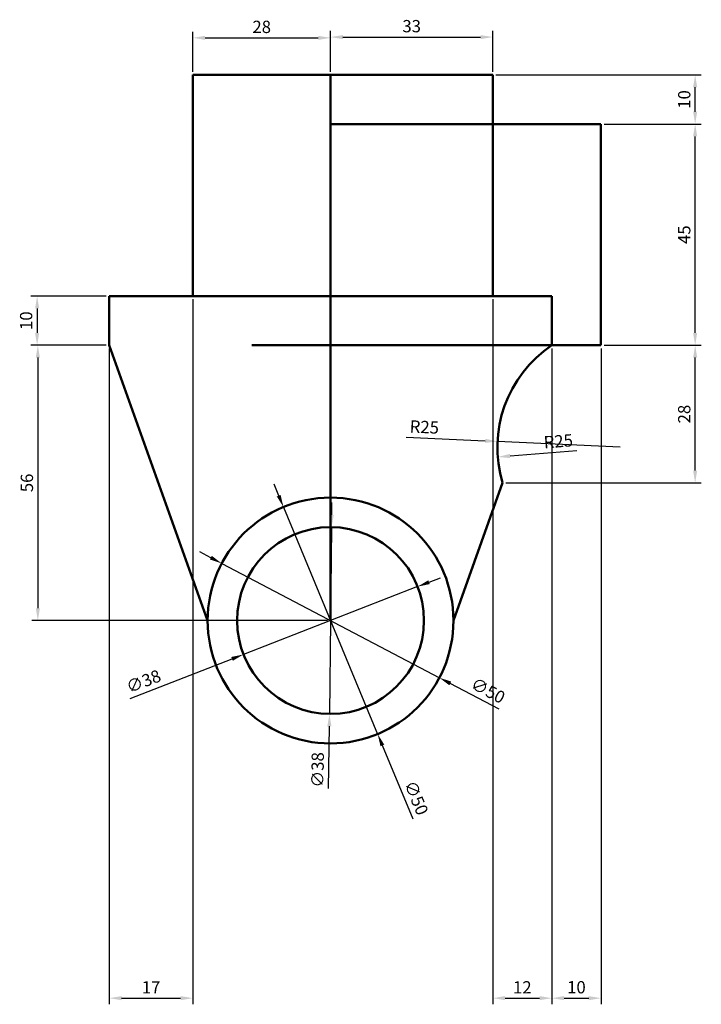
# Model space of a CAD drawing. Units: millimetres. Extents: x 2172 to 2566, y 897 to 1244.
# Tile 3 of 3: x 2427 to 2566, y 906 to 1106. Entities that reach past the tile are written whole.
import ezdxf

# ---------------------------------------------------------------- set-up
doc = ezdxf.new("R2010")
doc.units = ezdxf.units.MM
doc.layers.add('M-DIMS', color=2, linetype='Continuous', lineweight=25)
doc.layers.add('M-OUTL', color=7, linetype='Continuous', lineweight=50)
doc.styles.get("Standard").update_dxf_attribs({"font": 'arial.ttf'})
doc.dimstyles.new('ISO-25', dxfattribs={"dimtxt": 2.5, "dimasz": 2.5, "dimexe": 1.25, "dimexo": 0.625, "dimtad": 1, "dimtxsty": 'Standard', "dimcen": 2.5, "dimadec": 0, "dimazin": 0, "dimtfac": 1, "dimtmove": 0, "dimatfit": 3, "dimfxl": 1, "dimarcsym": 0})

# ---------------------------------------------------------------- blocks, each defined once
blk = doc.blocks.new('*D3')
at = {"layer": 'Defpoints', "color": 0, "transparency": 16777216}
for p in [(2507.9, 990.53), (2472.49, 976.73)]:
    blk.add_point(p, dxfattribs=at)
at = {"layer": 'M-DIMS', "color": 0, "lineweight": -2, "transparency": 16777216}
for p, q in [((2510.23, 991.43), (2512.56, 992.34)), ((2507.9, 990.53), (2472.49, 976.73)), ((2449.48, 967.76), (2470.16, 975.82))]:
    blk.add_line(p, q, dxfattribs=at)
at = {"layer": 'M-DIMS', "color": 0, "transparency": 16777216}
for points in [[(2510.08, 991.82), (2510.38, 991.05), (2507.9, 990.53)], [(2470.01, 976.21), (2470.32, 975.44), (2472.49, 976.73)]]:
    blk.add_solid(points, dxfattribs=at)
at = {"layer": 'M-DIMS', "color": 0, "transparency": 16777216, "insert": (2452.28, 970.97), "char_height": 2.5, "attachment_point": 5, "rotation": 21.2859}
blk.add_mtext('∅38', dxfattribs=at)
blk = doc.blocks.new('*D4')
at = {"layer": 'Defpoints', "color": 0, "transparency": 16777216}
for p in [(2468.07, 995.25), (2512.33, 972)]:
    blk.add_point(p, dxfattribs=at)
at = {"layer": 'M-DIMS', "color": 0, "lineweight": -2, "transparency": 16777216}
for p, q in [((2465.85, 996.42), (2463.64, 997.58)), ((2468.07, 995.25), (2512.33, 972)), ((2524.5, 965.61), (2514.54, 970.84))]:
    blk.add_line(p, q, dxfattribs=at)
at = {"layer": 'M-DIMS', "color": 0, "transparency": 16777216}
for points in [[(2466.05, 996.79), (2465.66, 996.05), (2468.07, 995.25)], [(2514.74, 971.21), (2514.35, 970.47), (2512.33, 972)]]:
    blk.add_solid(points, dxfattribs=at)
at = {"layer": 'M-DIMS', "color": 0, "transparency": 16777216, "insert": (2522.08, 969.11), "char_height": 2.5, "attachment_point": 5, "rotation": 332.2866}
blk.add_mtext('∅50', dxfattribs=at)
blk = doc.blocks.new('*D5')
at = {"layer": 'Defpoints', "color": 0, "transparency": 16777216}
for p in [(2549.13, 1018.87), (2524.2, 1016.9)]:
    blk.add_point(p, dxfattribs=at)
at = {"layer": 'M-DIMS', "color": 0, "lineweight": -2, "transparency": 16777216}
blk.add_line((2540.29, 1018.17), (2526.7, 1017.1), dxfattribs=at)
at = {"layer": 'M-DIMS', "color": 0, "transparency": 16777216}
blk.add_solid([(2526.66, 1017.51), (2526.73, 1016.68), (2524.2, 1016.9)], dxfattribs=at)
at = {"layer": 'M-DIMS', "color": 0, "transparency": 16777216, "insert": (2536.54, 1019.78), "char_height": 2.5, "attachment_point": 5, "rotation": 4.5166}
blk.add_mtext('R25', dxfattribs=at)
blk = doc.blocks.new('*D6')
at = {"layer": 'Defpoints', "color": 0, "transparency": 16777216}
for p in [(2445.2, 1039.63), (2430.67, 983.63), (2490.2, 983.63)]:
    blk.add_point(p, dxfattribs=at)
at = {"layer": 'M-DIMS', "color": 0, "lineweight": -2, "transparency": 16777216}
for p, q in [((2444.57, 1039.63), (2429.42, 1039.63)), ((2430.67, 1037.13), (2430.67, 986.13)), ((2489.57, 983.63), (2429.42, 983.63))]:
    blk.add_line(p, q, dxfattribs=at)
at = {"layer": 'M-DIMS', "color": 0, "transparency": 16777216}
for points in [[(2430.26, 1037.13), (2431.09, 1037.13), (2430.67, 1039.63)], [(2430.26, 986.13), (2431.09, 986.13), (2430.67, 983.63)]]:
    blk.add_solid(points, dxfattribs=at)
at = {"layer": 'M-DIMS', "color": 0, "transparency": 16777216, "insert": (2428.77, 1011.63), "char_height": 2.5, "attachment_point": 5, "rotation": 90}
blk.add_mtext('56', dxfattribs=at)
blk = doc.blocks.new('*D7')
at = {"layer": 'Defpoints', "color": 0, "transparency": 16777216}
for p in [(2445.2, 1049.63), (2430.53, 1039.63), (2445.2, 1039.63)]:
    blk.add_point(p, dxfattribs=at)
at = {"layer": 'M-DIMS', "color": 0, "lineweight": -2, "transparency": 16777216}
for p, q in [((2444.57, 1049.63), (2429.28, 1049.63)), ((2430.53, 1047.13), (2430.53, 1042.13)), ((2444.57, 1039.63), (2429.28, 1039.63))]:
    blk.add_line(p, q, dxfattribs=at)
at = {"layer": 'M-DIMS', "color": 0, "transparency": 16777216}
for points in [[(2430.11, 1047.13), (2430.94, 1047.13), (2430.53, 1049.63)], [(2430.11, 1042.13), (2430.94, 1042.13), (2430.53, 1039.63)]]:
    blk.add_solid(points, dxfattribs=at)
at = {"layer": 'M-DIMS', "color": 0, "transparency": 16777216, "insert": (2428.62, 1044.63), "char_height": 2.5, "attachment_point": 5, "rotation": 90}
blk.add_mtext('10', dxfattribs=at)
blk = doc.blocks.new('*D8')
at = {"layer": 'Defpoints', "color": 0, "transparency": 16777216}
for p in [(2490.2, 1102.17), (2462.2, 1094.63), (2490.2, 1094.63)]:
    blk.add_point(p, dxfattribs=at)
at = {"layer": 'M-DIMS', "color": 0, "lineweight": -2, "transparency": 16777216}
for p, q in [((2462.2, 1095.25), (2462.2, 1103.42)), ((2464.7, 1102.17), (2487.7, 1102.17)), ((2490.2, 1095.25), (2490.2, 1103.42))]:
    blk.add_line(p, q, dxfattribs=at)
at = {"layer": 'M-DIMS', "color": 0, "transparency": 16777216}
for points in [[(2464.7, 1102.58), (2464.7, 1101.75), (2462.2, 1102.17)], [(2487.7, 1102.58), (2487.7, 1101.75), (2490.2, 1102.17)]]:
    blk.add_solid(points, dxfattribs=at)
at = {"layer": 'M-DIMS', "color": 0, "transparency": 16777216, "insert": (2476.2, 1104.07), "char_height": 2.5, "attachment_point": 5}
blk.add_mtext('28', dxfattribs=at)
blk = doc.blocks.new('*D9')
at = {"layer": 'Defpoints', "color": 0, "transparency": 16777216}
for p in [(2523.2, 1102.32), (2490.2, 1094.63), (2523.2, 1094.63)]:
    blk.add_point(p, dxfattribs=at)
at = {"layer": 'M-DIMS', "color": 0, "lineweight": -2, "transparency": 16777216}
for p, q in [((2490.2, 1095.25), (2490.2, 1103.57)), ((2492.7, 1102.32), (2520.7, 1102.32)), ((2523.2, 1095.25), (2523.2, 1103.57))]:
    blk.add_line(p, q, dxfattribs=at)
at = {"layer": 'M-DIMS', "color": 0, "transparency": 16777216}
for points in [[(2492.7, 1102.73), (2492.7, 1101.9), (2490.2, 1102.32)], [(2520.7, 1102.73), (2520.7, 1101.9), (2523.2, 1102.32)]]:
    blk.add_solid(points, dxfattribs=at)
at = {"layer": 'M-DIMS', "color": 0, "transparency": 16777216, "insert": (2506.7, 1104.22), "char_height": 2.5, "attachment_point": 5}
blk.add_mtext('33', dxfattribs=at)
blk = doc.blocks.new('*D55')
at = {"layer": 'Defpoints', "color": 0, "transparency": 16777216}
for p in [(2462.2, 1049.63), (2445.2, 1039.63), (2462.2, 906.81)]:
    blk.add_point(p, dxfattribs=at)
at = {"layer": 'M-DIMS', "color": 0, "lineweight": -2, "transparency": 16777216}
for p, q in [((2462.2, 1049), (2462.2, 905.56)), ((2445.2, 1039), (2445.2, 905.56)), ((2447.7, 906.81), (2459.7, 906.81))]:
    blk.add_line(p, q, dxfattribs=at)
at = {"layer": 'M-DIMS', "color": 0, "transparency": 16777216}
for points in [[(2447.7, 907.23), (2447.7, 906.4), (2445.2, 906.81)], [(2459.7, 907.23), (2459.7, 906.4), (2462.2, 906.81)]]:
    blk.add_solid(points, dxfattribs=at)
at = {"layer": 'M-DIMS', "color": 0, "transparency": 16777216, "insert": (2453.7, 908.69), "char_height": 2.5, "attachment_point": 5}
blk.add_mtext('17', dxfattribs=at)
blk = doc.blocks.new('*D56')
at = {"layer": 'Defpoints', "color": 0, "transparency": 16777216}
for p in [(2523.2, 1049.63), (2535.2, 1039.63), (2535.2, 906.81)]:
    blk.add_point(p, dxfattribs=at)
at = {"layer": 'M-DIMS', "color": 0, "lineweight": -2, "transparency": 16777216}
for p, q in [((2523.2, 1049), (2523.2, 905.56)), ((2535.2, 1039), (2535.2, 905.56)), ((2525.7, 906.81), (2532.7, 906.81))]:
    blk.add_line(p, q, dxfattribs=at)
at = {"layer": 'M-DIMS', "color": 0, "transparency": 16777216}
for points in [[(2525.7, 907.23), (2525.7, 906.4), (2523.2, 906.81)], [(2532.7, 907.23), (2532.7, 906.4), (2535.2, 906.81)]]:
    blk.add_solid(points, dxfattribs=at)
at = {"layer": 'M-DIMS', "color": 0, "transparency": 16777216, "insert": (2529.2, 908.69), "char_height": 2.5, "attachment_point": 5}
blk.add_mtext('12', dxfattribs=at)
blk = doc.blocks.new('*D57')
at = {"layer": 'Defpoints', "color": 0, "transparency": 16777216}
for p in [(2535.2, 1039.63), (2545.2, 1039.63), (2545.2, 906.81)]:
    blk.add_point(p, dxfattribs=at)
at = {"layer": 'M-DIMS', "color": 0, "lineweight": -2, "transparency": 16777216}
for p, q in [((2535.2, 1039), (2535.2, 905.56)), ((2545.2, 1039), (2545.2, 905.56)), ((2537.7, 906.81), (2542.7, 906.81))]:
    blk.add_line(p, q, dxfattribs=at)
at = {"layer": 'M-DIMS', "color": 0, "transparency": 16777216}
for points in [[(2537.7, 907.23), (2537.7, 906.4), (2535.2, 906.81)], [(2542.7, 907.23), (2542.7, 906.4), (2545.2, 906.81)]]:
    blk.add_solid(points, dxfattribs=at)
at = {"layer": 'M-DIMS', "color": 0, "transparency": 16777216, "insert": (2540.2, 908.71), "char_height": 2.5, "attachment_point": 5}
blk.add_mtext('10', dxfattribs=at)
blk = doc.blocks.new('*D58')
at = {"layer": 'Defpoints', "color": 0, "transparency": 16777216}
for p in [(2545.2, 1039.63), (2564.35, 1039.63), (2525.2, 1011.63)]:
    blk.add_point(p, dxfattribs=at)
at = {"layer": 'M-DIMS', "color": 0, "lineweight": -2, "transparency": 16777216}
for p, q in [((2545.82, 1039.63), (2565.6, 1039.63)), ((2564.35, 1014.13), (2564.35, 1037.13)), ((2525.82, 1011.63), (2565.6, 1011.63))]:
    blk.add_line(p, q, dxfattribs=at)
at = {"layer": 'M-DIMS', "color": 0, "transparency": 16777216}
for points in [[(2563.93, 1037.13), (2564.76, 1037.13), (2564.35, 1039.63)], [(2563.93, 1014.13), (2564.76, 1014.13), (2564.35, 1011.63)]]:
    blk.add_solid(points, dxfattribs=at)
at = {"layer": 'M-DIMS', "color": 0, "transparency": 16777216, "insert": (2562.45, 1025.63), "char_height": 2.5, "attachment_point": 5, "rotation": 90}
blk.add_mtext('28', dxfattribs=at)
blk = doc.blocks.new('*D59')
at = {"layer": 'Defpoints', "color": 0, "transparency": 16777216}
for p in [(2545.2, 1084.63), (2564.35, 1084.63), (2545.2, 1039.63)]:
    blk.add_point(p, dxfattribs=at)
at = {"layer": 'M-DIMS', "color": 0, "lineweight": -2, "transparency": 16777216}
for p, q in [((2545.82, 1084.63), (2565.6, 1084.63)), ((2564.35, 1042.13), (2564.35, 1082.13)), ((2545.82, 1039.63), (2565.6, 1039.63))]:
    blk.add_line(p, q, dxfattribs=at)
at = {"layer": 'M-DIMS', "color": 0, "transparency": 16777216}
for points in [[(2563.93, 1082.13), (2564.76, 1082.13), (2564.35, 1084.63)], [(2563.93, 1042.13), (2564.76, 1042.13), (2564.35, 1039.63)]]:
    blk.add_solid(points, dxfattribs=at)
at = {"layer": 'M-DIMS', "color": 0, "transparency": 16777216, "insert": (2562.45, 1062.13), "char_height": 2.5, "attachment_point": 5, "rotation": 90}
blk.add_mtext('45', dxfattribs=at)
blk = doc.blocks.new('*D60')
at = {"layer": 'Defpoints', "color": 0, "transparency": 16777216}
for p in [(2523.2, 1094.63), (2564.35, 1094.63), (2545.2, 1084.63)]:
    blk.add_point(p, dxfattribs=at)
at = {"layer": 'M-DIMS', "color": 0, "lineweight": -2, "transparency": 16777216}
for p, q in [((2523.82, 1094.63), (2565.6, 1094.63)), ((2564.35, 1087.13), (2564.35, 1092.13)), ((2545.82, 1084.63), (2565.6, 1084.63))]:
    blk.add_line(p, q, dxfattribs=at)
at = {"layer": 'M-DIMS', "color": 0, "transparency": 16777216}
for points in [[(2563.93, 1092.13), (2564.76, 1092.13), (2564.35, 1094.63)], [(2563.93, 1087.13), (2564.76, 1087.13), (2564.35, 1084.63)]]:
    blk.add_solid(points, dxfattribs=at)
at = {"layer": 'M-DIMS', "color": 0, "transparency": 16777216, "insert": (2562.45, 1089.63), "char_height": 2.5, "attachment_point": 5, "rotation": 90}
blk.add_mtext('10', dxfattribs=at)
blk = doc.blocks.new('*D71')
at = {"layer": 'Defpoints', "color": 0, "transparency": 16777216}
for p in [(2480.62, 1006.72), (2499.78, 960.54)]:
    blk.add_point(p, dxfattribs=at)
at = {"layer": 'M-DIMS', "color": 0, "lineweight": -2, "transparency": 16777216}
for p, q in [((2479.66, 1009.03), (2478.7, 1011.34)), ((2480.62, 1006.72), (2499.78, 960.54)), ((2506.97, 943.2), (2500.74, 958.23))]:
    blk.add_line(p, q, dxfattribs=at)
at = {"layer": 'M-DIMS', "color": 0, "transparency": 16777216}
for points in [[(2480.04, 1009.19), (2479.27, 1008.87), (2480.62, 1006.72)], [(2501.12, 958.39), (2500.35, 958.07), (2499.78, 960.54)]]:
    blk.add_solid(points, dxfattribs=at)
at = {"layer": 'M-DIMS', "color": 0, "transparency": 16777216, "insert": (2507.35, 947.44), "char_height": 2.5, "attachment_point": 5, "rotation": 292.5319}
blk.add_mtext('∅50', dxfattribs=at)
blk = doc.blocks.new('*D72')
at = {"layer": 'Defpoints', "color": 0, "transparency": 16777216}
for p in [(2490.41, 1002.63), (2489.98, 964.63)]:
    blk.add_point(p, dxfattribs=at)
at = {"layer": 'M-DIMS', "color": 0, "lineweight": -2, "transparency": 16777216}
for p, q in [((2490.44, 1005.13), (2490.47, 1007.63)), ((2490.41, 1002.63), (2489.98, 964.63)), ((2489.81, 949.45), (2489.96, 962.13))]:
    blk.add_line(p, q, dxfattribs=at)
at = {"layer": 'M-DIMS', "color": 0, "transparency": 16777216}
for points in [[(2490.02, 1005.13), (2490.85, 1005.12), (2490.41, 1002.63)], [(2489.54, 962.13), (2490.37, 962.13), (2489.98, 964.63)]]:
    blk.add_solid(points, dxfattribs=at)
at = {"layer": 'M-DIMS', "color": 0, "transparency": 16777216, "insert": (2487.89, 953.25), "char_height": 2.5, "attachment_point": 5, "rotation": 89.359}
blk.add_mtext('∅38', dxfattribs=at)
blk = doc.blocks.new('*D73')
at = {"layer": 'Defpoints', "color": 0, "transparency": 16777216}
for p in [(2524.15, 1020.06), (2549.13, 1018.87)]:
    blk.add_point(p, dxfattribs=at)
at = {"layer": 'M-DIMS', "color": 0, "lineweight": -2, "transparency": 16777216}
for p, q in [((2505.55, 1020.96), (2521.66, 1020.18)), ((2549.13, 1018.87), (2524.15, 1020.06))]:
    blk.add_line(p, q, dxfattribs=at)
at = {"layer": 'M-DIMS', "color": 0, "transparency": 16777216}
blk.add_solid([(2521.68, 1020.6), (2521.64, 1019.77), (2524.15, 1020.06)], dxfattribs=at)
at = {"layer": 'M-DIMS', "color": 0, "transparency": 16777216, "insert": (2509.26, 1022.68), "char_height": 2.5, "attachment_point": 5, "rotation": 357.2579}
blk.add_mtext('R25', dxfattribs=at)

msp = doc.modelspace()

# ---------------------------------------------------------------- linework, layer by layer
at = {"layer": 'M-OUTL'}
for p, q in [((2462.1972, 1049.6287), (2462.1972, 1094.6287)), ((2462.1972, 1094.6287), (2490.1972, 1094.6287)), ((2490.1972, 1094.6287), (2490.1972, 1049.6287)), ((2523.1972, 1094.6287), (2490.1972, 1094.6287)), ((2523.1972, 1049.6287), (2523.1972, 1094.6287)), ((2545.1972, 1084.6287), (2490.1972, 1084.6287)), ((2545.1972, 1039.6287), (2545.1972, 1084.6287)), ((2445.1972, 1049.6287), (2535.1972, 1049.6287)), ((2445.1972, 1049.6287), (2445.1972, 1039.6287)), ((2490.1972, 1049.6287), (2462.1972, 1049.6287)), ((2490.1972, 1049.6287), (2490.1972, 983.6287)), ((2490.1972, 1049.6287), (2523.1972, 1049.6287)), ((2535.1972, 1049.6287), (2535.1972, 1039.6287)), ((2465.1972, 983.6287), (2445.1972, 1039.6287)), ((2535.1972, 1039.6287), (2474.1823, 1039.6287)), ((2535.1972, 1039.6287), (2545.1972, 1039.6287)), ((2515.1972, 983.6287), (2525.1972, 1011.6287)), ((2490.1972, 983.6287), (2490.1972, 983.6287))]:
    msp.add_line(p, q, dxfattribs=at)
for radius in [25, 19]:
    msp.add_circle((2490.1972, 983.6287), radius, dxfattribs=at)
msp.add_arc((2549.126, 1018.8684), 25, 123.859007, 196.833345, dxfattribs=at)

# ---------------------------------------------------------------- dimensions: what is measured, and where the dimension line sits
at = {"layer": 'M-DIMS'}
for base, p1, p2, override, picture, middle in [((2490.1972, 1102.1679), (2462.1972, 1094.6287), (2490.1972, 1094.6287), {"dimclrd": 0, "dimclre": 0, "dimclrt": 0}, '*D8', (2476.1972, 1104.0693)), ((2523.1972, 1102.3162), (2490.1972, 1094.6287), (2523.1972, 1094.6287), {"dimclrd": 0, "dimclre": 0, "dimclrt": 0}, '*D9', (2506.6972, 1104.2185)), ((2462.1972, 906.8126), (2445.1972, 1039.6287), (2462.1972, 1049.6287), {"dimdec": 0, "dimlfac": 1, "dimrnd": 0, "dimzin": 0, "dimdsep": 46, "dimlunit": 2}, '*D55', (2453.6972, 908.6927)), ((2535.1972, 906.8126), (2523.1972, 1049.6287), (2535.1972, 1039.6287), {"dimdec": 0, "dimlfac": 1, "dimrnd": 0, "dimzin": 0, "dimdsep": 46, "dimlunit": 2}, '*D56', (2529.1972, 908.6927)), ((2545.1972, 906.8126), (2535.1972, 1039.6287), (2545.1972, 1039.6287), {"dimdec": 0, "dimlfac": 1, "dimrnd": 0, "dimzin": 0, "dimdsep": 46, "dimlunit": 2}, '*D57', (2540.1972, 908.714))]:
    dim = msp.add_linear_dim(base=base, p1=p1, p2=p2, dimstyle='ISO-25', override=override, dxfattribs=at)
    dim.commit()
    dim.dimension.update_dxf_attribs({"geometry": picture, "text_midpoint": middle})
for base, p1, p2, override, picture, middle in [((2564.3472, 1094.6287), (2545.1972, 1084.6287), (2523.1972, 1094.6287), {"dimdec": 0, "dimlfac": 1, "dimrnd": 0, "dimzin": 0, "dimdsep": 46, "dimlunit": 2}, '*D60', (2562.4458, 1089.6287)), ((2564.3472, 1084.6287), (2545.1972, 1039.6287), (2545.1972, 1084.6287), {"dimdec": 0, "dimlfac": 1, "dimrnd": 0, "dimzin": 0, "dimdsep": 46, "dimlunit": 2}, '*D59', (2562.4509, 1062.1287)), ((2430.5251, 1039.6287), (2445.1972, 1049.6287), (2445.1972, 1039.6287), {"dimclrd": 0, "dimclre": 0, "dimclrt": 0}, '*D7', (2428.6237, 1044.6287)), ((2430.673, 983.6287), (2445.1972, 1039.6287), (2490.1972, 983.6287), {"dimclrd": 0, "dimclre": 0, "dimclrt": 0}, '*D6', (2428.7716, 1011.6287)), ((2564.3472, 1039.6287), (2525.1972, 1011.6287), (2545.1972, 1039.6287), {"dimdec": 0, "dimlfac": 1, "dimrnd": 0, "dimzin": 0, "dimdsep": 46, "dimlunit": 2}, '*D58', (2562.4458, 1025.6287))]:
    dim = msp.add_linear_dim(base=base, p1=p1, p2=p2, angle=90, dimstyle='ISO-25', override=override, dxfattribs=at)
    dim.commit()
    dim.dimension.update_dxf_attribs({"geometry": picture, "text_midpoint": middle})
for mpoint, override, picture, middle in [((2524.1546, 1020.0644), {"dimdec": 0, "dimlfac": 1, "dimrnd": 0, "dimzin": 0, "dimdsep": 46, "dimlunit": 2}, '*D73', (2509.1718, 1020.782)), ((2524.2036, 1016.8997), {"dimclrd": 0, "dimclre": 0, "dimclrt": 0}, '*D5', (2536.6849, 1017.8857))]:
    dim = msp.add_radius_dim(center=(2549.126, 1018.8684), mpoint=mpoint, dimstyle='ISO-25', override=override, dxfattribs=at)
    dim.commit()
    dim.dimension.update_dxf_attribs({"geometry": picture, "text_midpoint": middle, "dimtype": 164})
for p1, p2, override, picture, middle in [((2480.6173, 1006.7204), (2499.7772, 960.5371), {"dimdec": 0, "dimlfac": 1, "dimrnd": 0, "dimzin": 0, "dimdsep": 46, "dimlunit": 2}, '*D71', (2505.5252, 946.6821)), ((2490.4098, 1002.6275), (2489.9847, 964.6299), {"dimdec": 0, "dimlfac": 1, "dimrnd": 0, "dimzin": 0, "dimdsep": 46, "dimlunit": 2}, '*D72', (2489.8571, 953.2306)), ((2468.0651, 995.2549), (2512.3293, 972.0025), {"dimclrd": 0, "dimclre": 0, "dimclrt": 0}, '*D4', (2521.1601, 967.3636)), ((2507.9011, 990.5261), (2472.4934, 976.7313), {"dimclrd": 0, "dimclre": 0, "dimclrt": 0}, '*D3', (2452.9991, 969.1363))]:
    dim = msp.add_diameter_dim_2p(p1=p1, p2=p2, dimstyle='ISO-25', override=override, dxfattribs=at)
    dim.commit()
    dim.dimension.update_dxf_attribs({"geometry": picture, "text_midpoint": middle, "dimtype": 163})

doc.saveas('drawing.dxf')
